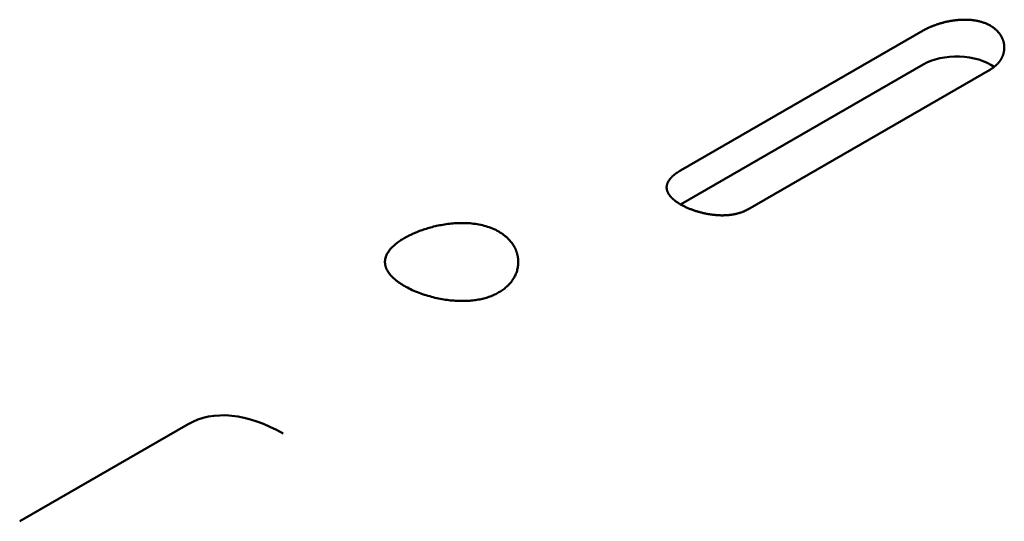
# Model space of a CAD drawing. Units: inches. Extents: x 105 to 6825, y 111 to 6061.
# Tile 2 of 2: x 3609 to 6825, y 4421 to 6061. Entities that reach past the tile are written whole.
import ezdxf

# ---------------------------------------------------------------- set-up
doc = ezdxf.new("R2010")
doc.units = ezdxf.units.IN
doc.header["$MEASUREMENT"] = 0
doc.layers.add('M-OUTL', color=7, linetype='Continuous', lineweight=50)

msp = doc.modelspace()

# ---------------------------------------------------------------- linework, layer by layer
at = {"layer": 'M-OUTL'}
for p, q in [((5767.7, 5567.7), (6559.6, 6024.9)), ((5767.7, 5456.8), (6559.6, 5914)), ((5987.7, 5440.7), (6779.6, 5897.9)), ((3608.9, 4420.8), (4158.8, 4738.3))]:
    msp.add_line(p, q, dxfattribs=at)
for points in [[(6779.6, 6041), (6777.4, 6042.3), (6775.1, 6043.5), (6772.8, 6044.6), (6770.5, 6045.8), (6768.1, 6046.8), (6765.7, 6047.9), (6763.3, 6048.9), (6760.8, 6049.9), (6758.3, 6050.8), (6755.8, 6051.6), (6753.3, 6052.5), (6750.7, 6053.3), (6748.1, 6054), (6745.5, 6054.7), (6742.9, 6055.4), (6740.3, 6056), (6737.7, 6056.6), (6735, 6057.1), (6732.4, 6057.6), (6729.7, 6058.1), (6727.1, 6058.5), (6724.4, 6058.8), (6721.7, 6059.2), (6719.1, 6059.5), (6716.4, 6059.8), (6713.7, 6060), (6711.1, 6060.2), (6708.4, 6060.4), (6705.8, 6060.5), (6703.1, 6060.6), (6700.5, 6060.7), (6697.9, 6060.7), (6695.2, 6060.7), (6692.6, 6060.7), (6690, 6060.6), (6687.4, 6060.6), (6684.8, 6060.4), (6682.2, 6060.3), (6679.6, 6060.2), (6677.1, 6060), (6674.5, 6059.8), (6672, 6059.5), (6669.5, 6059.3), (6667, 6059), (6664.5, 6058.7), (6662, 6058.4), (6659.6, 6058.1), (6657.1, 6057.7), (6654.7, 6057.4), (6652.2, 6057), (6649.8, 6056.5), (6647.4, 6056.1), (6645.1, 6055.7), (6642.7, 6055.2), (6640.4, 6054.7), (6638, 6054.2), (6635.7, 6053.7), (6633.4, 6053.2), (6631.2, 6052.6), (6628.9, 6052.1), (6626.6, 6051.5), (6624.4, 6050.9), (6622.2, 6050.3), (6620, 6049.7), (6617.8, 6049.1), (6615.7, 6048.5), (6613.5, 6047.8), (6611.4, 6047.2), (6609.3, 6046.5), (6607.2, 6045.8), (6605.1, 6045.1), (6603.1, 6044.4), (6601, 6043.7), (6599, 6043), (6597, 6042.2), (6595, 6041.5), (6593.1, 6040.7), (6591.1, 6040), (6589.2, 6039.2), (6587.3, 6038.4), (6585.4, 6037.6), (6583.6, 6036.8), (6581.7, 6036), (6579.9, 6035.2), (6578.1, 6034.4), (6576.3, 6033.6), (6574.5, 6032.7), (6572.8, 6031.9), (6571.1, 6031), (6569.4, 6030.2), (6567.7, 6029.3), (6566, 6028.4), (6564.4, 6027.6), (6562.8, 6026.7), (6561.2, 6025.8), (6559.6, 6024.9)], [(6825.2, 5969.5), (6825.2, 5970.3), (6825.1, 5971), (6825.1, 5971.8), (6825.1, 5972.6), (6825.1, 5973.4), (6825, 5974.1), (6825, 5974.9), (6824.9, 5975.7), (6824.8, 5976.5), (6824.7, 5977.2), (6824.7, 5978), (6824.6, 5978.8), (6824.4, 5979.6), (6824.3, 5980.4), (6824.2, 5981.2), (6824.1, 5982), (6823.9, 5982.8), (6823.8, 5983.5), (6823.6, 5984.3), (6823.4, 5985.1), (6823.3, 5985.9), (6823.1, 5986.7), (6822.9, 5987.5), (6822.7, 5988.3), (6822.5, 5989.1), (6822.2, 5989.9), (6822, 5990.7), (6821.7, 5991.5), (6821.5, 5992.3), (6821.2, 5993.1), (6820.9, 5993.9), (6820.7, 5994.7), (6820.4, 5995.5), (6820.1, 5996.3), (6819.7, 5997.1), (6819.4, 5997.9), (6819.1, 5998.7), (6818.7, 5999.4), (6818.4, 6000.2), (6818, 6001), (6817.6, 6001.8), (6817.2, 6002.6), (6816.8, 6003.4), (6816.4, 6004.2), (6816, 6005), (6815.6, 6005.8), (6815.1, 6006.6), (6814.7, 6007.3), (6814.2, 6008.1), (6813.7, 6008.9), (6813.2, 6009.7), (6812.7, 6010.5), (6812.2, 6011.2), (6811.7, 6012), (6811.2, 6012.8), (6810.6, 6013.6), (6810.1, 6014.3), (6809.5, 6015.1), (6808.9, 6015.9), (6808.3, 6016.6), (6807.7, 6017.4), (6807.1, 6018.1), (6806.5, 6018.9), (6805.8, 6019.6), (6805.2, 6020.4), (6804.5, 6021.1), (6803.8, 6021.9), (6803.2, 6022.6), (6802.5, 6023.3), (6801.8, 6024.1), (6801, 6024.8), (6800.3, 6025.5), (6799.6, 6026.2), (6798.8, 6026.9), (6798.1, 6027.6), (6797.3, 6028.3), (6796.5, 6029), (6795.7, 6029.7), (6794.9, 6030.4), (6794.1, 6031), (6793.2, 6031.7), (6792.4, 6032.4), (6791.6, 6033), (6790.7, 6033.7), (6789.8, 6034.3), (6788.9, 6035), (6788.1, 6035.6), (6787.2, 6036.2), (6786.2, 6036.9), (6785.3, 6037.5), (6784.4, 6038.1), (6783.5, 6038.7), (6782.5, 6039.3), (6781.5, 6039.9), (6780.6, 6040.4), (6779.6, 6041)], [(6779.6, 5897.9), (6780.5, 5898.4), (6781.3, 5898.9), (6782.2, 5899.4), (6783, 5899.9), (6783.8, 5900.4), (6784.6, 5901), (6785.5, 5901.5), (6786.3, 5902), (6787.1, 5902.6), (6787.9, 5903.1), (6788.7, 5903.7), (6789.4, 5904.3), (6790.2, 5904.8), (6791, 5905.4), (6791.8, 5906), (6792.5, 5906.6), (6793.3, 5907.2), (6794, 5907.8), (6794.7, 5908.4), (6795.4, 5909), (6796.2, 5909.6), (6796.9, 5910.2), (6797.6, 5910.9), (6798.3, 5911.5), (6799, 5912.1), (6799.6, 5912.8), (6800.3, 5913.4), (6801, 5914.1), (6801.6, 5914.7), (6802.3, 5915.4), (6802.9, 5916.1), (6803.5, 5916.7), (6804.2, 5917.4), (6804.8, 5918.1), (6805.4, 5918.8), (6806, 5919.5), (6806.6, 5920.2), (6807.2, 5920.9), (6807.7, 5921.6), (6808.3, 5922.3), (6808.9, 5923), (6809.4, 5923.8), (6810, 5924.5), (6810.5, 5925.2), (6811, 5926), (6811.5, 5926.7), (6812.1, 5927.5), (6812.6, 5928.2), (6813, 5929), (6813.5, 5929.7), (6814, 5930.5), (6814.5, 5931.3), (6814.9, 5932.1), (6815.4, 5932.9), (6815.8, 5933.6), (6816.2, 5934.4), (6816.7, 5935.2), (6817.1, 5936), (6817.5, 5936.8), (6817.9, 5937.7), (6818.2, 5938.5), (6818.6, 5939.3), (6819, 5940.1), (6819.3, 5940.9), (6819.7, 5941.8), (6820, 5942.6), (6820.3, 5943.5), (6820.7, 5944.3), (6821, 5945.2), (6821.3, 5946), (6821.5, 5946.9), (6821.8, 5947.7), (6822.1, 5948.6), (6822.3, 5949.5), (6822.6, 5950.3), (6822.8, 5951.2), (6823, 5952.1), (6823.2, 5953), (6823.4, 5953.9), (6823.6, 5954.8), (6823.8, 5955.7), (6824, 5956.6), (6824.1, 5957.5), (6824.3, 5958.4), (6824.4, 5959.3), (6824.6, 5960.2), (6824.7, 5961.1), (6824.8, 5962), (6824.9, 5963), (6824.9, 5963.9), (6825, 5964.8), (6825.1, 5965.7), (6825.1, 5966.7), (6825.1, 5967.6), (6825.2, 5968.6), (6825.2, 5969.5)], [(5767.7, 5567.7), (5766.9, 5567.2), (5766, 5566.7), (5765.2, 5566.2), (5764.3, 5565.7), (5763.5, 5565.2), (5762.7, 5564.7), (5761.9, 5564.1), (5761.1, 5563.6), (5760.3, 5563.1), (5759.5, 5562.6), (5758.7, 5562.1), (5757.9, 5561.6), (5757.1, 5561.1), (5756.3, 5560.5), (5755.6, 5560), (5754.8, 5559.5), (5754.1, 5559), (5753.3, 5558.4), (5752.6, 5557.9), (5751.9, 5557.4), (5751.2, 5556.8), (5750.5, 5556.3), (5749.8, 5555.8), (5749.1, 5555.2), (5748.4, 5554.7), (5747.7, 5554.1), (5747, 5553.6), (5746.4, 5553.1), (5745.7, 5552.5), (5745.1, 5552), (5744.4, 5551.4), (5743.8, 5550.9), (5743.2, 5550.3), (5742.5, 5549.8), (5741.9, 5549.2), (5741.3, 5548.6), (5740.7, 5548.1), (5740.2, 5547.5), (5739.6, 5547), (5739, 5546.4), (5738.5, 5545.8), (5737.9, 5545.3), (5737.4, 5544.7), (5736.8, 5544.1), (5736.3, 5543.6), (5735.8, 5543), (5735.3, 5542.4), (5734.8, 5541.8), (5734.3, 5541.3), (5733.8, 5540.7), (5733.3, 5540.1), (5732.9, 5539.5), (5732.4, 5538.9), (5732, 5538.4), (5731.5, 5537.8), (5731.1, 5537.2), (5730.7, 5536.6), (5730.3, 5536), (5729.9, 5535.4), (5729.5, 5534.8), (5729.1, 5534.2), (5728.7, 5533.6), (5728.4, 5533), (5728, 5532.4), (5727.7, 5531.8), (5727.3, 5531.2), (5727, 5530.6), (5726.7, 5530), (5726.4, 5529.4), (5726.1, 5528.8), (5725.8, 5528.2), (5725.5, 5527.6), (5725.3, 5526.9), (5725, 5526.3), (5724.8, 5525.7), (5724.5, 5525.1), (5724.3, 5524.5), (5724.1, 5523.8), (5723.9, 5523.2), (5723.7, 5522.6), (5723.5, 5522), (5723.3, 5521.3), (5723.2, 5520.7), (5723, 5520.1), (5722.9, 5519.4), (5722.8, 5518.8), (5722.7, 5518.1), (5722.6, 5517.5), (5722.5, 5516.9), (5722.4, 5516.2), (5722.3, 5515.6), (5722.3, 5514.9), (5722.2, 5514.3), (5722.2, 5513.6), (5722.2, 5513), (5722.2, 5512.3)], [(5722.2, 5512.3), (5722.2, 5511.8), (5722.2, 5511.2), (5722.2, 5510.7), (5722.2, 5510.2), (5722.3, 5509.6), (5722.3, 5509.1), (5722.4, 5508.5), (5722.4, 5508), (5722.5, 5507.5), (5722.6, 5506.9), (5722.7, 5506.4), (5722.8, 5505.8), (5722.9, 5505.3), (5723, 5504.7), (5723.1, 5504.2), (5723.3, 5503.6), (5723.4, 5503.1), (5723.6, 5502.5), (5723.7, 5501.9), (5723.9, 5501.4), (5724.1, 5500.8), (5724.3, 5500.3), (5724.5, 5499.7), (5724.7, 5499.1), (5724.9, 5498.6), (5725.1, 5498), (5725.3, 5497.4), (5725.6, 5496.9), (5725.8, 5496.3), (5726.1, 5495.7), (5726.4, 5495.2), (5726.7, 5494.6), (5727, 5494), (5727.3, 5493.4), (5727.6, 5492.9), (5727.9, 5492.3), (5728.3, 5491.7), (5728.6, 5491.1), (5729, 5490.6), (5729.3, 5490), (5729.7, 5489.4), (5730.1, 5488.8), (5730.5, 5488.2), (5730.9, 5487.6), (5731.3, 5487), (5731.8, 5486.5), (5732.2, 5485.9), (5732.7, 5485.3), (5733.1, 5484.7), (5733.6, 5484.1), (5734.1, 5483.5), (5734.6, 5482.9), (5735.1, 5482.3), (5735.6, 5481.7), (5736.2, 5481.1), (5736.7, 5480.5), (5737.3, 5479.9), (5737.8, 5479.3), (5738.4, 5478.7), (5739, 5478.1), (5739.6, 5477.5), (5740.2, 5476.9), (5740.9, 5476.3), (5741.5, 5475.7), (5742.2, 5475.1), (5742.8, 5474.5), (5743.5, 5473.9), (5744.2, 5473.3), (5744.9, 5472.7), (5745.6, 5472.1), (5746.3, 5471.5), (5747, 5470.9), (5747.8, 5470.3), (5748.5, 5469.7), (5749.3, 5469.1), (5750.1, 5468.5), (5750.8, 5467.9), (5751.6, 5467.3), (5752.4, 5466.7), (5753.3, 5466.1), (5754.1, 5465.5), (5754.9, 5464.9), (5755.8, 5464.4), (5756.6, 5463.8), (5757.5, 5463.2), (5758.4, 5462.6), (5759.3, 5462), (5760.2, 5461.4), (5761.1, 5460.8), (5762, 5460.3), (5762.9, 5459.7), (5763.9, 5459.1), (5764.8, 5458.5), (5765.8, 5457.9), (5766.8, 5457.4), (5767.7, 5456.8)], [(5767.7, 5456.8), (5770, 5455.5), (5772.2, 5454.3), (5774.5, 5453.1), (5776.8, 5451.9), (5779.2, 5450.7), (5781.6, 5449.5), (5784, 5448.3), (5786.5, 5447.2), (5789, 5446), (5791.5, 5444.9), (5794.1, 5443.9), (5796.6, 5442.8), (5799.2, 5441.8), (5801.8, 5440.8), (5804.4, 5439.8), (5807, 5438.8), (5809.7, 5437.9), (5812.3, 5436.9), (5815, 5436.1), (5817.6, 5435.2), (5820.3, 5434.4), (5822.9, 5433.5), (5825.6, 5432.8), (5828.3, 5432), (5830.9, 5431.3), (5833.6, 5430.6), (5836.2, 5429.9), (5838.9, 5429.2), (5841.6, 5428.6), (5844.2, 5428), (5846.8, 5427.4), (5849.5, 5426.9), (5852.1, 5426.3), (5854.7, 5425.8), (5857.3, 5425.4), (5859.9, 5424.9), (5862.5, 5424.5), (5865.1, 5424.1), (5867.7, 5423.7), (5870.2, 5423.4), (5872.8, 5423.1), (5875.3, 5422.8), (5877.8, 5422.5), (5880.3, 5422.2), (5882.8, 5422), (5885.3, 5421.8), (5887.8, 5421.7), (5890.2, 5421.5), (5892.7, 5421.4), (5895.1, 5421.3), (5897.5, 5421.2), (5899.9, 5421.1), (5902.3, 5421.1), (5904.6, 5421.1), (5907, 5421.1), (5909.3, 5421.2), (5911.6, 5421.2), (5913.9, 5421.3), (5916.2, 5421.4), (5918.4, 5421.5), (5920.7, 5421.7), (5922.9, 5421.9), (5925.1, 5422.1), (5927.3, 5422.3), (5929.5, 5422.5), (5931.7, 5422.8), (5933.8, 5423.1), (5935.9, 5423.4), (5938.1, 5423.7), (5940.1, 5424.1), (5942.2, 5424.5), (5944.3, 5424.9), (5946.3, 5425.3), (5948.3, 5425.7), (5950.3, 5426.2), (5952.3, 5426.7), (5954.3, 5427.2), (5956.2, 5427.7), (5958.1, 5428.2), (5960, 5428.8), (5961.9, 5429.4), (5963.8, 5430), (5965.6, 5430.6), (5967.4, 5431.3), (5969.2, 5432), (5971, 5432.7), (5972.8, 5433.4), (5974.5, 5434.1), (5976.3, 5434.9), (5978, 5435.6), (5979.6, 5436.4), (5981.3, 5437.2), (5982.9, 5438.1), (5984.5, 5438.9), (5986.1, 5439.8), (5987.7, 5440.7)], [(5173.8, 5367.9), (5169, 5370.6), (5164, 5373.2), (5158.9, 5375.6), (5153.7, 5377.9), (5148.3, 5380), (5142.9, 5382), (5137.4, 5383.9), (5131.8, 5385.6), (5126.2, 5387.2), (5120.5, 5388.6), (5114.8, 5389.9), (5109, 5391.1), (5103.2, 5392.1), (5097.4, 5393), (5091.6, 5393.8), (5085.8, 5394.4), (5080, 5395), (5074.3, 5395.4), (5068.5, 5395.7), (5062.7, 5395.9), (5057, 5396), (5051.3, 5396), (5045.7, 5395.9), (5040, 5395.7), (5034.4, 5395.4), (5028.9, 5395.1), (5023.3, 5394.6), (5017.9, 5394.1), (5012.4, 5393.5), (5007.1, 5392.8), (5001.7, 5392.1), (4996.4, 5391.3), (4991.2, 5390.5), (4986, 5389.5), (4980.9, 5388.6), (4975.8, 5387.5), (4970.8, 5386.4), (4965.8, 5385.3), (4960.9, 5384.1), (4956.1, 5382.9), (4951.3, 5381.6), (4946.6, 5380.3), (4941.9, 5378.9), (4937.3, 5377.5), (4932.7, 5376), (4928.2, 5374.5), (4923.8, 5373), (4919.4, 5371.5), (4915.1, 5369.9), (4910.9, 5368.2), (4906.7, 5366.6), (4902.6, 5364.9), (4898.5, 5363.2), (4894.6, 5361.4), (4890.7, 5359.7), (4886.8, 5357.9), (4883.1, 5356), (4879.4, 5354.2), (4875.7, 5352.3), (4872.2, 5350.4), (4868.7, 5348.5), (4865.3, 5346.5), (4861.9, 5344.6), (4858.7, 5342.6), (4855.5, 5340.6), (4852.4, 5338.5), (4849.4, 5336.5), (4846.4, 5334.4), (4843.5, 5332.3), (4840.8, 5330.2), (4838.1, 5328.1), (4835.4, 5325.9), (4832.9, 5323.7), (4830.5, 5321.5), (4828.1, 5319.3), (4825.8, 5317.1), (4823.7, 5314.9), (4821.6, 5312.6), (4819.6, 5310.3), (4817.7, 5308), (4815.9, 5305.7), (4814.2, 5303.4), (4812.6, 5301), (4811.1, 5298.6), (4809.7, 5296.2), (4808.4, 5293.8), (4807.3, 5291.4), (4806.2, 5288.9), (4805.3, 5286.5), (4804.4, 5284), (4803.7, 5281.4), (4803.1, 5278.9), (4802.7, 5276.4), (4802.3, 5273.8), (4802.1, 5271.2), (4802.1, 5268.6)], [(5237.6, 5268.6), (5237.6, 5269.6), (5237.6, 5270.7), (5237.5, 5271.8), (5237.5, 5272.8), (5237.5, 5273.9), (5237.4, 5275), (5237.3, 5276), (5237.2, 5277.1), (5237.1, 5278.2), (5237, 5279.3), (5236.9, 5280.4), (5236.8, 5281.5), (5236.6, 5282.5), (5236.4, 5283.6), (5236.3, 5284.7), (5236.1, 5285.8), (5235.9, 5286.9), (5235.7, 5288), (5235.4, 5289.1), (5235.2, 5290.2), (5235, 5291.3), (5234.7, 5292.4), (5234.4, 5293.5), (5234.1, 5294.6), (5233.8, 5295.7), (5233.5, 5296.8), (5233.2, 5297.9), (5232.8, 5299), (5232.5, 5300.1), (5232.1, 5301.2), (5231.7, 5302.3), (5231.3, 5303.4), (5230.9, 5304.5), (5230.5, 5305.6), (5230, 5306.7), (5229.6, 5307.8), (5229.1, 5308.9), (5228.6, 5310), (5228.1, 5311.2), (5227.6, 5312.3), (5227, 5313.4), (5226.5, 5314.5), (5225.9, 5315.6), (5225.4, 5316.7), (5224.8, 5317.7), (5224.2, 5318.8), (5223.5, 5319.9), (5222.9, 5321), (5222.2, 5322.1), (5221.6, 5323.2), (5220.9, 5324.3), (5220.2, 5325.4), (5219.5, 5326.4), (5218.7, 5327.5), (5218, 5328.6), (5217.2, 5329.7), (5216.4, 5330.7), (5215.6, 5331.8), (5214.8, 5332.9), (5214, 5333.9), (5213.2, 5335), (5212.3, 5336), (5211.4, 5337.1), (5210.5, 5338.1), (5209.6, 5339.1), (5208.7, 5340.2), (5207.8, 5341.2), (5206.8, 5342.2), (5205.8, 5343.2), (5204.8, 5344.2), (5203.8, 5345.3), (5202.8, 5346.3), (5201.8, 5347.2), (5200.7, 5348.2), (5199.7, 5349.2), (5198.6, 5350.2), (5197.5, 5351.1), (5196.4, 5352.1), (5195.2, 5353.1), (5194.1, 5354), (5192.9, 5354.9), (5191.7, 5355.9), (5190.6, 5356.8), (5189.4, 5357.7), (5188.1, 5358.6), (5186.9, 5359.5), (5185.7, 5360.4), (5184.4, 5361.2), (5183.1, 5362.1), (5181.8, 5363), (5180.5, 5363.8), (5179.2, 5364.7), (5177.9, 5365.5), (5176.5, 5366.3), (5175.2, 5367.1), (5173.8, 5367.9)], [(4802.1, 5268.6), (4802.1, 5267.8), (4802.1, 5267), (4802.1, 5266.3), (4802.2, 5265.5), (4802.2, 5264.8), (4802.3, 5264), (4802.4, 5263.2), (4802.4, 5262.5), (4802.5, 5261.7), (4802.7, 5260.9), (4802.8, 5260.1), (4802.9, 5259.4), (4803.1, 5258.6), (4803.2, 5257.8), (4803.4, 5257), (4803.6, 5256.2), (4803.8, 5255.4), (4804, 5254.7), (4804.2, 5253.9), (4804.5, 5253.1), (4804.7, 5252.3), (4805, 5251.5), (4805.3, 5250.7), (4805.5, 5249.9), (4805.9, 5249.1), (4806.2, 5248.3), (4806.5, 5247.5), (4806.8, 5246.7), (4807.2, 5245.9), (4807.6, 5245.1), (4808, 5244.2), (4808.4, 5243.4), (4808.8, 5242.6), (4809.2, 5241.8), (4809.7, 5241), (4810.1, 5240.2), (4810.6, 5239.3), (4811.1, 5238.5), (4811.6, 5237.7), (4812.1, 5236.9), (4812.6, 5236), (4813.2, 5235.2), (4813.7, 5234.4), (4814.3, 5233.5), (4814.9, 5232.7), (4815.5, 5231.9), (4816.1, 5231), (4816.8, 5230.2), (4817.4, 5229.4), (4818.1, 5228.5), (4818.8, 5227.7), (4819.5, 5226.9), (4820.2, 5226), (4820.9, 5225.2), (4821.7, 5224.3), (4822.4, 5223.5), (4823.2, 5222.6), (4824, 5221.8), (4824.8, 5220.9), (4825.7, 5220.1), (4826.5, 5219.3), (4827.4, 5218.4), (4828.2, 5217.6), (4829.1, 5216.7), (4830, 5215.9), (4831, 5215), (4831.9, 5214.2), (4832.9, 5213.3), (4833.8, 5212.5), (4834.8, 5211.6), (4835.8, 5210.8), (4836.9, 5209.9), (4837.9, 5209.1), (4839, 5208.2), (4840, 5207.4), (4841.1, 5206.5), (4842.2, 5205.7), (4843.3, 5204.9), (4844.4, 5204), (4845.6, 5203.2), (4846.8, 5202.4), (4847.9, 5201.5), (4849.1, 5200.7), (4850.3, 5199.9), (4851.5, 5199), (4852.8, 5198.2), (4854, 5197.4), (4855.3, 5196.6), (4856.6, 5195.7), (4857.8, 5194.9), (4859.1, 5194.1), (4860.5, 5193.3), (4861.8, 5192.5), (4863.1, 5191.7), (4864.5, 5190.9), (4865.9, 5190.1)], [(4865.9, 5190.1), (4870.7, 5187.4), (4875.7, 5184.7), (4880.8, 5182.1), (4886, 5179.5), (4891.3, 5177), (4896.8, 5174.6), (4902.3, 5172.2), (4907.9, 5170), (4913.5, 5167.8), (4919.2, 5165.6), (4924.9, 5163.6), (4930.7, 5161.7), (4936.5, 5159.8), (4942.3, 5158.1), (4948.1, 5156.4), (4953.9, 5154.8), (4959.7, 5153.3), (4965.4, 5151.9), (4971.2, 5150.6), (4977, 5149.4), (4982.7, 5148.2), (4988.4, 5147.2), (4994.1, 5146.2), (4999.7, 5145.3), (5005.3, 5144.5), (5010.9, 5143.8), (5016.4, 5143.2), (5021.8, 5142.7), (5027.3, 5142.2), (5032.7, 5141.8), (5038, 5141.5), (5043.3, 5141.3), (5048.5, 5141.2), (5053.7, 5141.1), (5058.8, 5141.2), (5063.9, 5141.3), (5068.9, 5141.4), (5073.9, 5141.7), (5078.8, 5142), (5083.6, 5142.4), (5088.4, 5142.9), (5093.2, 5143.5), (5097.8, 5144.1), (5102.5, 5144.8), (5107, 5145.6), (5111.5, 5146.5), (5115.9, 5147.4), (5120.3, 5148.4), (5124.6, 5149.4), (5128.9, 5150.6), (5133, 5151.8), (5137.1, 5153), (5141.2, 5154.4), (5145.2, 5155.8), (5149.1, 5157.3), (5152.9, 5158.8), (5156.7, 5160.4), (5160.4, 5162.1), (5164, 5163.8), (5167.6, 5165.6), (5171, 5167.5), (5174.4, 5169.4), (5177.8, 5171.4), (5181, 5173.5), (5184.2, 5175.6), (5187.3, 5177.8), (5190.3, 5180.1), (5193.3, 5182.4), (5196.2, 5184.7), (5198.9, 5187.2), (5201.6, 5189.6), (5204.3, 5192.2), (5206.8, 5194.8), (5209.2, 5197.4), (5211.6, 5200.2), (5213.9, 5202.9), (5216, 5205.8), (5218.1, 5208.6), (5220.1, 5211.6), (5222, 5214.6), (5223.8, 5217.6), (5225.5, 5220.7), (5227.1, 5223.8), (5228.6, 5227), (5230, 5230.2), (5231.2, 5233.5), (5232.4, 5236.8), (5233.5, 5240.2), (5234.4, 5243.6), (5235.2, 5247.1), (5235.9, 5250.6), (5236.5, 5254.1), (5237, 5257.7), (5237.3, 5261.3), (5237.5, 5264.9), (5237.6, 5268.6)]]:
    msp.add_lwpolyline(points, dxfattribs=at)
for centre, major_axis, start_param, end_param in [((6669.6, 5850.5), (-155.5, 0), 3.808511, 5.497787), ((4469.9, 4199.5), (311.1, -538.8), 2.356194, 3.141593)]:
    msp.add_ellipse(centre, major_axis=major_axis, ratio=0.57735, start_param=start_param, end_param=end_param, dxfattribs=at)

doc.saveas('drawing.dxf')
